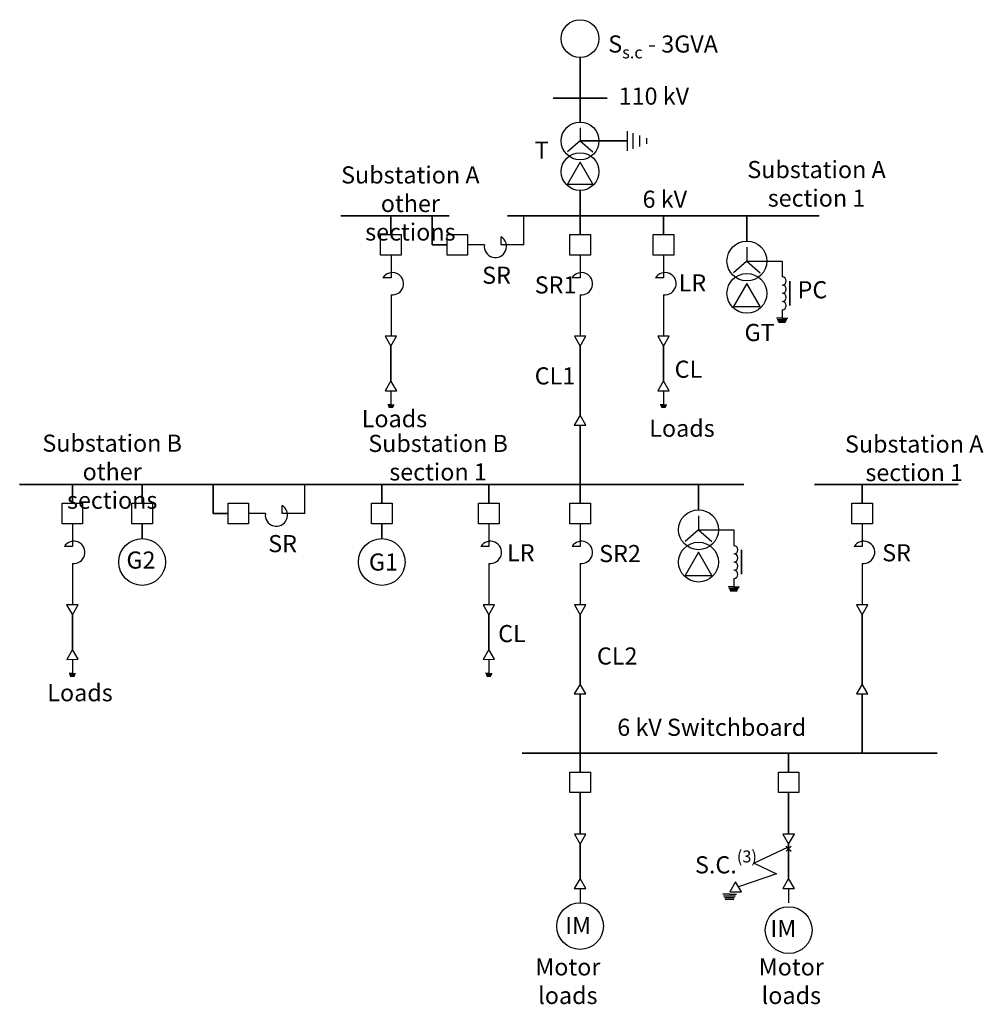
# Model space of a CAD drawing. Units: inches. Extents: x 197 to 309, y 89 to 204.
import ezdxf

# ---------------------------------------------------------------- set-up
doc = ezdxf.new("R2010")
doc.units = ezdxf.units.IN
doc.header["$MEASUREMENT"] = 0
for name, color, linetype, lineweight in [('E-ANNO-TEXT', 3, 'Continuous', 18), ('E-EQPM', 4, 'Continuous', 25), ('E-ONEL', 7, 'Continuous', 35)]:
    doc.layers.add(name, color=color, linetype=linetype, lineweight=lineweight)
doc.styles.get("Standard").update_dxf_attribs({"font": 'arial.ttf'})

# ---------------------------------------------------------------- blocks, each defined once
blk = doc.blocks.new('E-BREAKER')
blk.add_lwpolyline([(0, 2.4), (2.4, 2.4), (2.4, 0), (0, 0)], close=True)
blk = doc.blocks.new('E-CABLE-TERM')
blk.add_lwpolyline([(0, 1.16), (0.67, 0), (1.34, 1.16)], close=True)
blk = doc.blocks.new('E-REACTOR')
for p, q in [((0.94, 9.47), (0.94, 6.82)), ((0.94, 6.82), (0, 6.82)), ((0.94, 4.85), (0.94, 0))]:
    blk.add_line(p, q)
blk.add_arc((1.11, 6.14), 1.3, 262.2765, 148.4768)
blk = doc.blocks.new('E-REACTOR-SECT')
for p, q in [((6.58, 1.48), (6.58, 4.88)), ((3.94, 1.48), (3.94, 2.42)), ((1.96, 1.48), (0, 1.48)), ((6.58, 1.48), (3.94, 1.48))]:
    blk.add_line(p, q)
blk.add_arc((3.25, 1.3), 1.3, 172.2765, 58.4768)
blk = doc.blocks.new('E-GROUND')
for p, q in [((0.38, 1.66), (0.38, 0)), ((0.38, 0), (0, 0)), ((0.38, 0), (0.76, 0))]:
    blk.add_line(p, q)
blk = doc.blocks.new('E-XFMR-GROUNDING')
for p, q in [((2.33, 8.28), (2.33, 6.66)), ((2.33, 6.66), (0.77, 5.3)), ((2.33, 6.66), (3.89, 5.3)), ((2.33, 6.66), (6.45, 6.66)), ((6.45, 6.66), (6.45, 4.8)), ((6.45, 0.97), (6.45, 0)), ((6.45, 0), (5.8, 0)), ((6.45, 0), (7.1, 0))]:
    blk.add_line(p, q)
blk.add_lwpolyline([(3.89, 1.33), (2.33, 4.04), (0.77, 1.33)], close=True)
for centre in [(2.33, 6.66), (2.33, 2.88)]:
    blk.add_circle(centre, 2.33)
for centre in [(6.45, 4.32), (6.45, 3.37), (6.45, 2.41), (6.45, 1.45)]:
    blk.add_arc(centre, 0.478, 270, 90)

msp = doc.modelspace()

# ---------------------------------------------------------------- linework, layer by layer
at = {"layer": 'E-EQPM'}
for p, q in [((262.06, 191.31), (262.06, 190.03)), ((262.06, 190.03), (262.06, 189.78)), ((267.61, 188.63), (267.61, 190.93)), ((268.26, 188.86), (268.26, 190.7)), ((268.26, 188.86), (268.26, 190.7)), ((269.06, 189.14), (269.06, 190.41)), ((269.87, 189.43), (269.87, 190.12)), ((262.06, 189.78), (260.58, 188.5)), ((262.06, 189.78), (263.54, 188.5)), ((285.1, 168.93), (286.23, 168.93)), ((285.18, 168.77), (286.15, 168.77)), ((285.26, 168.6), (286.07, 168.6)), ((239.63, 158.85), (240.3, 158.85)), ((271.47, 158.85), (272.14, 158.85)), ((239.68, 158.75), (240.25, 158.75)), ((239.72, 158.66), (240.2, 158.66)), ((271.52, 158.75), (272.09, 158.75)), ((271.57, 158.66), (272.04, 158.66)), ((279.45, 137.53), (280.59, 137.53)), ((279.53, 137.37), (280.51, 137.37)), ((279.61, 137.21), (280.43, 137.21)), ((202.41, 127.45), (203.08, 127.45)), ((202.46, 127.36), (203.03, 127.36)), ((202.5, 127.26), (202.98, 127.26)), ((251.07, 127.45), (251.74, 127.45)), ((251.12, 127.36), (251.69, 127.36)), ((251.16, 127.26), (251.64, 127.26)), ((286.28, 107.22), (282.39, 105.38)), ((286.43, 107.07), (286.14, 107.36)), ((286.43, 107.07), (286.14, 106.78)), ((286.43, 107.07), (286.72, 107.36)), ((286.43, 107.07), (286.72, 106.78)), ((282.39, 105.38), (285.02, 104.15)), ((285.02, 104.15), (280.56, 102.63)), ((262.06, 102.43), (262.06, 100.77)), ((286.43, 102.43), (286.43, 100.77)), ((279.52, 101.77), (278.73, 101.77)), ((278.83, 101.57), (280.22, 101.57)), ((278.93, 101.37), (280.12, 101.37)), ((279.52, 101.77), (280.32, 101.77)), ((279.03, 101.17), (280.02, 101.17))]:
    msp.add_line(p, q, dxfattribs=at)
msp.add_lwpolyline([(263.54, 184.74), (262.06, 187.3), (260.58, 184.74)], close=True, dxfattribs=at)
for centre, radius in [((262.06, 201.74), 2.21), ((262.06, 189.78), 2.21), ((262.06, 186.2), 2.21), ((210.89, 140.58), 2.73), ((238.89, 140.58), 2.73), ((262.06, 98.04), 2.73), ((286.43, 97.57), 2.73)]:
    msp.add_circle(centre, radius, dxfattribs=at)
at = {"layer": 'E-ONEL'}
for p, q in [((262.06, 199.54), (262.06, 194.78)), ((262.06, 194.78), (258.9, 194.78)), ((262.06, 194.78), (265.21, 194.78)), ((262.06, 194.78), (262.06, 191.98)), ((262.06, 189.78), (267.61, 189.78)), ((262.06, 184), (262.06, 181.04)), ((242.56, 181.04), (234.1, 181.04)), ((239.96, 181.04), (239.96, 178.84)), ((246.77, 181.04), (242.56, 181.04)), ((244.77, 177.64), (244.77, 181.04)), ((262.06, 181.04), (253.58, 181.04)), ((262.06, 181.04), (281.55, 181.04)), ((262.06, 181.04), (262.06, 178.84)), ((271.8, 181.04), (271.8, 178.84)), ((281.55, 181.04), (290.01, 181.04)), ((281.55, 181.04), (281.55, 178.08)), ((246.52, 177.64), (244.77, 177.64)), ((286.58, 170.54), (286.58, 173.41)), ((239.96, 165.8), (239.96, 161.76)), ((262.06, 165.8), (262.06, 157.72)), ((271.8, 165.8), (271.8, 161.76)), ((262.06, 156.56), (262.06, 149.64)), ((196.58, 149.64), (281.2, 149.64)), ((202.74, 149.64), (202.74, 147.44)), ((210.89, 149.64), (210.89, 147.44)), ((219.18, 146.24), (219.18, 149.64)), ((238.89, 149.64), (238.89, 147.44)), ((251.4, 149.64), (251.4, 147.44)), ((262.06, 149.64), (262.06, 147.44)), ((275.91, 149.64), (275.91, 146.68)), ((289.45, 149.64), (306.22, 149.64)), ((295.01, 149.64), (295.01, 147.44)), ((220.93, 146.24), (219.18, 146.24)), ((210.89, 145.04), (210.89, 143.31)), ((238.89, 145.04), (238.89, 143.31)), ((280.93, 139.15), (280.93, 142.02)), ((202.74, 134.41), (202.74, 130.36)), ((251.4, 134.41), (251.4, 130.36)), ((262.06, 134.41), (262.06, 126.32)), ((295.01, 134.41), (295.01, 126.32)), ((262.06, 125.16), (262.06, 118.24)), ((295.01, 125.16), (295.01, 118.24)), ((255.31, 118.24), (303.79, 118.24)), ((262.06, 118.24), (262.06, 116.05)), ((286.43, 118.24), (286.43, 116.05)), ((262.06, 113.64), (262.06, 108.79)), ((286.43, 113.64), (286.43, 108.79)), ((262.06, 107.63), (262.06, 103.59)), ((286.43, 107.63), (286.43, 103.59))]:
    msp.add_line(p, q, dxfattribs=at)

# ---------------------------------------------------------------- block references
at = {"layer": 'E-EQPM'}
for name, p in [('E-REACTOR-SECT', (248.92, 176.16)), ('E-BREAKER', (238.76, 176.44)), ('E-BREAKER', (246.52, 176.44)), ('E-BREAKER', (260.86, 176.44)), ('E-BREAKER', (270.6, 176.44)), ('E-XFMR-GROUNDING', (279.22, 169.09)), ('E-REACTOR', (239.03, 166.96)), ('E-REACTOR', (261.12, 166.96)), ('E-REACTOR', (270.87, 166.96)), ('E-CABLE-TERM', (239.29, 165.8)), ('E-CABLE-TERM', (261.39, 165.8)), ('E-CABLE-TERM', (271.14, 165.8)), ('E-GROUND', (239.58, 158.94)), ('E-GROUND', (271.42, 158.94)), ('E-REACTOR-SECT', (223.33, 144.76)), ('E-BREAKER', (201.54, 145.04)), ('E-BREAKER', (209.69, 145.04)), ('E-BREAKER', (220.93, 145.04)), ('E-BREAKER', (237.69, 145.04)), ('E-BREAKER', (250.2, 145.04)), ('E-BREAKER', (260.86, 145.04)), ('E-BREAKER', (293.81, 145.04)), ('E-XFMR-GROUNDING', (273.57, 137.69)), ('E-REACTOR', (201.81, 135.57)), ('E-REACTOR', (250.47, 135.57)), ('E-REACTOR', (261.12, 135.57)), ('E-REACTOR', (294.08, 135.57)), ('E-CABLE-TERM', (202.07, 134.41)), ('E-CABLE-TERM', (250.73, 134.41)), ('E-CABLE-TERM', (261.39, 134.41)), ('E-CABLE-TERM', (294.35, 134.41)), ('E-GROUND', (202.36, 127.55)), ('E-GROUND', (251.02, 127.55)), ('E-BREAKER', (260.86, 113.64)), ('E-BREAKER', (285.23, 113.64)), ('E-CABLE-TERM', (261.39, 107.63)), ('E-CABLE-TERM', (285.76, 107.63))]:
    msp.add_blockref(name, p, dxfattribs=at)
for p, rotation in [((240.3, 160.02), 60.0000000000007), ((272.14, 160.02), 59.99999999999949), ((262.39, 155.98), 59.99999999999896), ((203.08, 128.63), 60.0000000000007), ((251.74, 128.63), 60.0000000000007), ((262.39, 124.58), 59.99999999999896), ((295.35, 124.58), 59.99999999999896), ((262.39, 101.85), 59.99999999999982), ((286.76, 101.85), 60.00000000000103), ((279.23, 102.62), 300.31158144789)]:
    msp.add_blockref('E-CABLE-TERM', p, dxfattribs=dict(at, rotation=rotation))

# ---------------------------------------------------------------- texts
at = {"layer": 'E-ANNO-TEXT', "char_height": 2, "attachment_point": 1}
for s, width, insert in [('\\A1;S{\\H0.7x;\\S^ s.c;} - 3GVA', 16.654, (265.35, 202.79)), ('110 kV', 10.1959, (266.57, 196.02)), ('T', 7.7462, (256.76, 189.7)), ('\\pxqc;Substation A\\Psection 1', 17.6004, (280.89, 187.44)), ('\\pxqc;Substation A\\Pother sections', 17.6004, (233.43, 186.81)), ('6 kV', 7.7462, (269.36, 183.97)), ('SR', 7.7462, (250.62, 175.09)), ('SR1', 7.7462, (256.76, 173.96)), ('LR', 7.7462, (273.58, 174.19)), ('PC', 7.7462, (287.48, 173.39)), ('GT', 7.7462, (281.27, 168.4)), ('CL', 7.7462, (273.11, 164.11)), ('CL1', 7.7462, (256.76, 163.33)), ('Loads', 7.7462, (236.55, 158.33)), ('Loads', 7.7462, (270.15, 157.21)), ('\\pxqc;Substation B\\Pother sections', 17.6004, (198.59, 155.47)), ('\\pxqc;Substation B\\Psection 1', 17.6004, (236.67, 155.44)), ('\\pxqc;Substation A\\Psection 1', 17.6004, (292.3, 155.37)), ('SR', 7.7462, (225.62, 143.73)), ('LR', 7.7462, (253.53, 142.66)), ('SR', 7.7462, (297.36, 142.66)), ('\\pxqc;G2', 7.7462, (206.88, 141.81)), ('G1', 7.7462, (237.39, 141.58)), ('SR2', 7.7462, (264.29, 142.57)), ('CL', 7.7462, (252.49, 133.22)), ('CL2', 7.7462, (264.03, 130.6)), ('Loads', 7.7462, (199.81, 126.31)), ('\\pxqc;6 kV Switchboard', 24.2077, (265.34, 122.27)), ('\\A1;S.C.{\\H0.7x;\\S(3)^ ;}', 7.7462, (275.49, 106.88)), ('IM', 7.7462, (260.33, 99.1)), ('IM', 7.7462, (284.3, 98.77)), ('\\pxqc;Motor\\Ploads', 7.7462, (256.76, 94.27)), ('\\pxqc;Motor\\Ploads', 7.7462, (282.87, 94.27))]:
    msp.add_mtext_dynamic_manual_height_columns(s, width=width, gutter_width=1, heights=[0], dxfattribs=dict(at, insert=insert))

doc.saveas('drawing.dxf')
